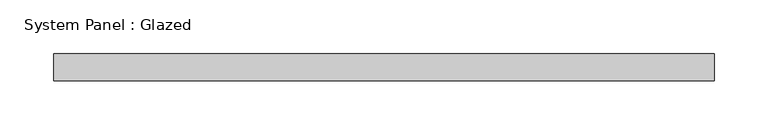
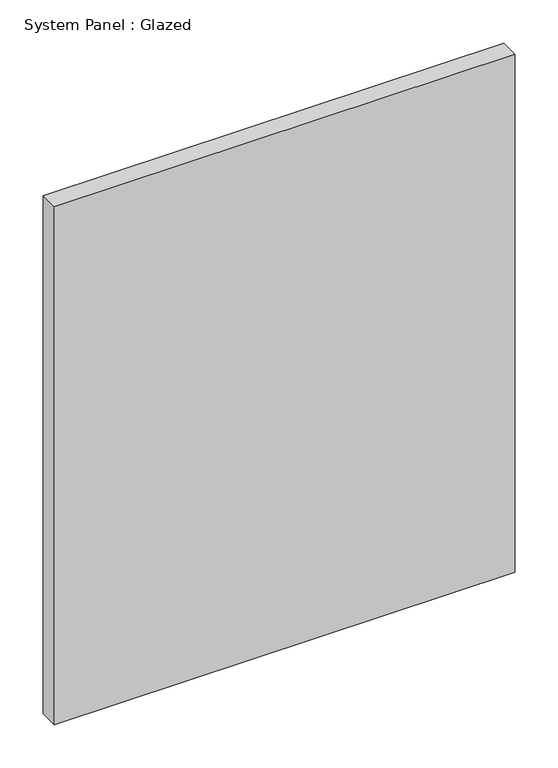
"""IFC4 building model written with IfcOpenShell, lengths in millimetres: plate geometry, System Panel : Glazed."""

from ifc_helpers import new_model, si_unit, origin, origin_with_axes, place, context, project, spatial, polyline, outline, extrude, source, transform, mapped, element, save


def system_panel_glazed_8a587fcc(model_context):
    return source(origin(), model_context, "Body", "SweptSolid", [
        extrude(outline(polyline([(307.975, 19.05), (-307.975, 19.05), (-307.975, 44.45), (307.975, 44.45), (307.975, 19.05)])), origin_with_axes(), (0.0, 0.0, 1.0), 732.0809713),
    ])


if __name__ == "__main__":
    model = new_model("IFC4")
    model_context = context("Model", 3, world=origin())
    ifc_project = project(units=[si_unit("LENGTHUNIT", "METRE", prefix="MILLI")], contexts=[model_context])
    site = spatial("IfcSite", under=ifc_project)
    building = spatial("IfcBuilding", under=site)
    placement = place(None, origin())
    system_panel_glazed_shape = system_panel_glazed_8a587fcc(model_context)
    element("IfcPlate", 1, ObjectType="System Panel : Glazed", at=placement, inside=building, context=model_context, shape_type="MappedRepresentation", body=[
        mapped(system_panel_glazed_shape, transform((0.0, 0.0, 0.0), x_axis=(1.0, 0.0, 0.0), y_axis=(0.0, 1.0, 0.0), z_axis=(0.0, 0.0, 1.0))),
    ])
    save(model, "model.ifc")

# Revit data of these elements
# Type "System Panel : Glazed"
#   Construction Type Id = "GSP4R"
#   Analytic Construction = "1/8 in Pilkington single glazing"
#   Visual Light Transmittance = 0.9
#   Solar Heat Gain Coefficient = 0.86
#   Heat Transfer Coefficient (U) = 1.18115 BTU/(h·ft²·°F)
#   Define Thermal Properties by = 1
# Element 1 (IfcPlate, "System Panel : Glazed")
#   Materials on its faces: "Glass"
# Materials
#   "Glass": class "Glass", colour RGB 0 128 192, transparency 0.75, Description = "Soda Lime Glass", Cost = 0
